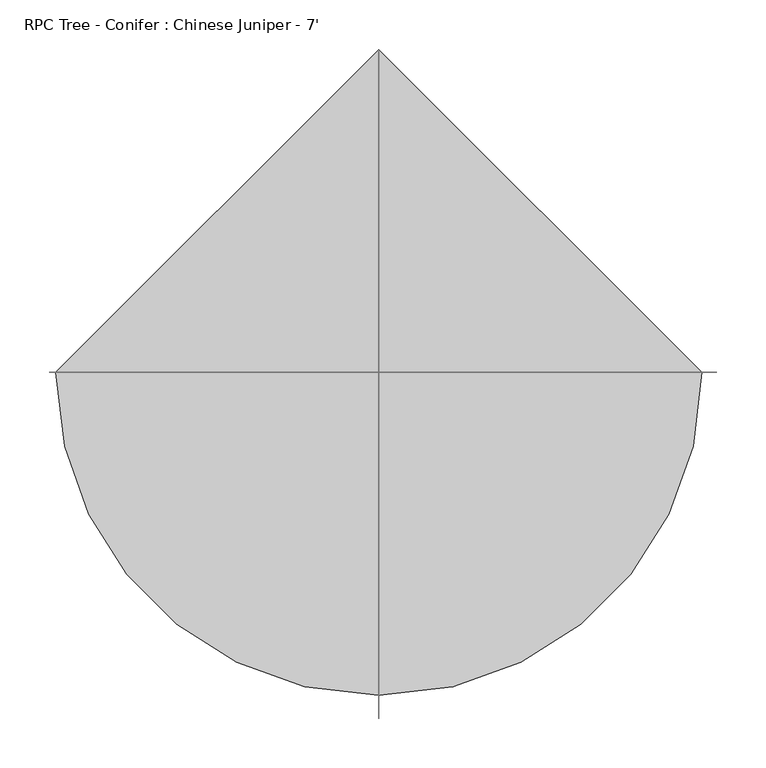
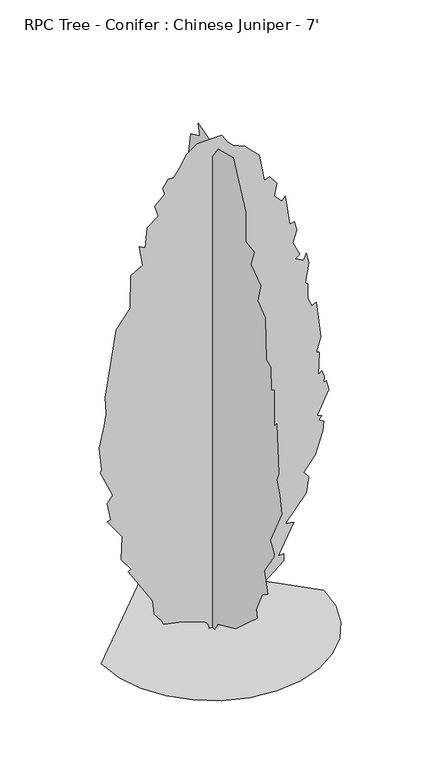
"""IFC4 building model written with IfcOpenShell, lengths in millimetres: geographic element geometry, RPC Tree - Conifer : Chinese Juniper - 7'."""

from ifc_helpers import new_model, si_unit, origin, place, context, project, spatial, triangles, source, transform, mapped, element, save


def rpc_tree_conifer_chinese_juniper_7_7598bbdc(model_context):
    return source(origin(), model_context, "Body", "Tessellation", [
        triangles([(-10.3135556, 5e-07, 9e-07), (-12.8060293, -2e-07, 12.8140684), (-19.5312093, -4e-07, 21.7081794), (-88.2070433, 1.1e-06, 46.9827109), (-143.9981418, 2.8e-06, 58.8213279), (-149.3455807, 2.2e-06, 72.1897524), (-170.8912042, 1.5e-06, 99.7706089), (-176.0828022, -7e-07, 141.7057854), (-184.1045146, -1.3e-06, 157.7479294), (-248.2723821, -4.6e-06, 259.3475236), (-239.9701817, -5.3e-06, 264.3368267), (-268.362017, -6.4e-06, 304.1387577), (-265.4845582, -1.07e-05, 374.7346484), (-309.7677564, -1.24e-05, 435.812788), (-299.0725335, -1.31e-05, 438.4852266), (-309.3523021, -1.58e-05, 492.5148502), (-293.7240046, -1.78e-05, 513.3483533), (-331.1564581, -2.11e-05, 596.2342461), (-325.8097278, -2.16e-05, 601.5809764), (-333.8307135, -2.56e-05, 673.7698477), (-319.3200076, -2.99e-05, 736.7529219), (-312.4402313, -3.24e-05, 772.6976755), (-315.1144867, -3.53e-05, 823.4978451), (-283.0305802, -4.87e-05, 1024.024268), (-242.9256517, -5.36e-05, 1077.4986929), (-240.7575791, -5.96e-05, 1177.3046648), (-205.4931982, -6.24e-05, 1197.8151861), (-216.1884393, -6.56e-05, 1259.3087437), (-197.9348478, -6.58e-05, 1248.8367085), (-192.1255003, -6.97e-05, 1310.1089859), (-160.0402858, -7.25e-05, 1334.1719067), (-170.7351817, -7.41e-05, 1368.9301048), (-141.3244133, -7.7e-05, 1395.667281), (-146.6718613, -7.79e-05, 1414.3835804), (-130.6297082, -8e-05, 1438.4465012), (-114.5875642, -8.07e-05, 1438.4465012), (-96.1815747, -8.29e-05, 1462.3443157), (-77.7287857, -8.58e-05, 1497.0336227), (-44.6214088, -8.86e-05, 1519.4527485), (26.5664902, -9.18e-05, 1520.5723022), (43.1603652, -9.1e-05, 1494.5933647), (59.2025137, -9.07e-05, 1478.551466), (94.8687642, -9.14e-05, 1463.445702), (136.7395278, -9.06e-05, 1419.7303471), (152.7816628, -8.64e-05, 1336.846162), (168.8238158, -8.74e-05, 1342.1929287), (188.3895002, -8.66e-05, 1314.20205), (182.191877, -8.41e-05, 1278.0250431), (203.5823773, -8.36e-05, 1253.9621223), (214.2758017, -8.47e-05, 1264.6573997), (227.6453163, -7.99e-05, 1173.7504486), (241.0130141, -8.06e-05, 1176.424704), (248.2828829, -7.94e-05, 1149.9378759), (236.3339574, -7.67e-05, 1113.592202), (257.0549855, -7.5e-05, 1069.4776709), (243.0450304, -7.39e-05, 1061.0775295), (267.7502266, -7.42e-05, 1048.0871887), (275.7712123, -7.56e-05, 1066.8034155), (283.792198, -7.41e-05, 1034.7194727), (273.0987737, -7.01e-05, 975.8983538), (280.8185786, -7.01e-05, 969.5464886), (279.746333, -6.74e-05, 926.116), (291.8131837, -6.63e-05, 898.3609354), (305.1827165, -6.72e-05, 903.7077021), (318.5503962, -6.11e-05, 791.4139023), (305.1827165, -5.8e-05, 748.6347548), (313.5084801, -5.81e-05, 745.8062937), (310.5294468, -5.39e-05, 676.4441031), (321.2246879, -5.48e-05, 684.4650524), (329.2456736, -5.41e-05, 665.7488256), (326.5713819, -5.28e-05, 647.0344156), (334.5923676, -5.33e-05, 649.7068542), (342.6133533, -5.19e-05, 620.2971668), (307.8551551, -4.63e-05, 550.7808068), (321.2246879, -4.65e-05, 545.4340765), (313.2037022, -4.56e-05, 534.7388354), (326.5713819, -4.57e-05, 526.7178497), (323.7592352, -4.38e-05, 497.9014764), (302.5084248, -3.89e-05, 430.4642409), (267.7502266, -3.48e-05, 387.6850571), (283.792198, -3.44e-05, 368.9688303), (275.0237288, -3.12e-05, 322.2617249), (214.2758017, -2.4e-05, 245.9798258), (238.3405755, -2.49e-05, 243.3055704), (192.8871181, -1.77e-05, 155.0742009), (208.9290895, -1.84e-05, 155.0742009), (208.9290895, -1.71e-05, 133.684618), (91.2864429, -6.2e-06, 37.4317359), (91.2864429, -7e-06, 50.8001605), (11.0759977, -5e-07, 0.0), (0.1966718, 9.8494079, 9.29e-05), (0.1966729, 24.6293697, 10.2116678), (0.1966747, 55.3021477, 21.3897713), (0.1966762, 127.4919001, 48.1266227), (0.1966794, 164.923636, 82.8846392), (0.1966788, 148.881492, 85.5583586), (0.1966849, 206.1035171, 168.0404152), (0.1966859, 188.9874833, 208.5473722), (0.1966882, 237.1133793, 278.0637686), (0.1966893, 231.7666672, 310.147675), (0.1966927, 266.5230486, 352.9268589), (0.1966955, 278.2089087, 404.0935395), (0.1966947, 271.8715775, 457.2014534), (0.1966993, 314.6507795, 521.369339), (0.1967023, 317.3232182, 585.539005), (0.1967039, 301.8799747, 638.0518244), (0.1967057, 325.3442039, 721.897506), (0.1967061, 303.9555203, 751.3071934), (0.1967086, 277.2183078, 836.8655611), (0.1967091, 295.9345346, 895.68668), (0.1967119, 274.5440343, 981.2450478), (0.196713, 247.8086386, 1032.0452173), (0.1967142, 234.439124, 1138.9940672), (0.1967132, 218.3971526, 1130.9731178), (0.1967174, 218.3971526, 1227.2249462), (0.1967163, 186.3132279, 1235.2458229), (0.1967152, 169.3394457, 1292.3597786), (0.1967168, 159.5761971, 1339.5204174), (0.1967168, 127.4919001, 1371.6043602), (0.1967204, 111.449747, 1467.8579327), (0.1967164, 65.9968483, 1489.2467434), (0.1967182, 72.8998653, 1523.6638287), (0.1967145, 8.1062543, 1503.0081127), (0.1967152, 4.5019648, 1457.1628006), (0.1967129, -27.5823121, 1502.6161308), (0.1967105, -105.1193285, 1524.0049416), (0.1967048, -169.2880862, 1392.9930256), (0.1967008, -169.2880862, 1302.0879639), (0.1966987, -211.5754214, 1294.5605164), (0.1966973, -193.3508616, 1245.9411003), (0.1966964, -244.8876323, 1210.7601809), (0.1966946, -230.7833333, 1155.0360386), (0.1966917, -268.2139701, 1125.6245344), (0.1966887, -273.562499, 997.2870192), (0.1966873, -295.3920532, 987.9742882), (0.1966841, -297.6254561, 917.0771622), (0.1966839, -313.6674093, 927.7706228), (0.1966819, -313.6674093, 815.4768957), (0.1966791, -327.0351254, 831.5188671), (0.196675, -337.7303664, 681.7926138), (0.1966744, -326.120719, 656.3254183), (0.1966719, -343.0789135, 617.6229115), (0.1966721, -351.0998629, 564.1485229), (0.1966695, -294.9511826, 449.1804677), (0.1966673, -313.6674093, 417.0965612), (0.1966698, -312.0853475, 405.769927), (0.1966688, -262.8672579, 334.2124489), (0.1966653, -281.5834847, 272.7170382), (0.1966657, -252.1719987, 254.0008115), (0.1966671, -222.7623476, 189.8329441), (0.1966658, -228.1090598, 165.7690968), (0.196666, -174.6353615, 117.6426557), (0.1966663, -118.4877531, 66.8424907), (0.1966685, -24.9082271, 24.0633114), (0.1966709, -11.5401454, 9.16e-05), (-327.063394, 0.0, 0.0001066), (-318.4110515, -74.9863023, 0.0001017), (-293.7711855, -143.8493682, 9.65e-05), (-255.1158779, -204.615799, 9.12e-05), (-204.4191359, -255.312541, 8.6e-05), (-143.652696, -293.9678487, 8.1e-05), (-74.7896301, -318.6077328, 7.66e-05), (0.1966858, -327.2600753, 7.28e-05), (75.1829745, -318.6077328, 7e-05), (144.0460404, -293.9678487, 6.85e-05), (204.8124621, -255.312541, 6.81e-05), (255.5092041, -204.615799, 6.89e-05), (294.1645118, -143.8491865, 7.08e-05), (318.8044141, -74.9863023, 7.39e-05), (327.4567566, 2.86e-05, 7.8e-05), (0.1966283, 327.2600753, 0.0001118)], [[57, 58, 59], [27, 28, 29], [87, 88, 89], [49, 50, 51], [13, 14, 15], [83, 84, 85], [74, 75, 76], [63, 64, 65], [68, 69, 70], [71, 72, 73], [9, 10, 11], [85, 86, 87], [85, 87, 89], [51, 52, 53], [54, 55, 56], [90, 1, 2], [66, 67, 68], [45, 46, 47], [17, 18, 19], [68, 70, 71], [45, 47, 48], [31, 32, 33], [76, 77, 78], [89, 90, 2], [89, 2, 3], [57, 59, 60], [51, 53, 54], [25, 26, 27], [39, 40, 41], [56, 57, 60], [71, 73, 74], [34, 35, 36], [33, 34, 36], [4, 5, 6], [60, 61, 62], [80, 81, 82], [38, 39, 41], [37, 38, 41], [37, 41, 42], [29, 30, 31], [15, 16, 17], [36, 37, 42], [33, 36, 42], [31, 33, 42], [31, 42, 43], [31, 43, 44], [31, 44, 45], [29, 31, 45], [29, 45, 48], [27, 29, 48], [25, 27, 48], [25, 48, 49], [25, 49, 51], [25, 51, 54], [25, 54, 56], [25, 56, 60], [25, 60, 62], [24, 25, 62], [23, 24, 62], [22, 23, 62], [22, 62, 63], [22, 63, 65], [22, 65, 66], [22, 66, 68], [21, 22, 68], [20, 21, 68], [19, 20, 68], [17, 19, 68], [17, 68, 71], [17, 71, 74], [15, 17, 74], [13, 15, 74], [13, 74, 76], [13, 76, 78], [13, 78, 79], [13, 79, 80], [12, 13, 80], [11, 12, 80], [9, 11, 80], [9, 80, 82], [9, 82, 83], [9, 83, 85], [9, 85, 89], [9, 89, 3], [9, 3, 4], [8, 9, 4], [8, 4, 6], [7, 8, 6], [138, 139, 140], [94, 95, 96], [136, 137, 138], [121, 122, 123], [112, 113, 114], [128, 129, 130], [121, 123, 124], [125, 126, 127], [124, 125, 127], [114, 115, 116], [147, 148, 149], [130, 131, 132], [124, 127, 128], [134, 135, 136], [154, 155, 91], [154, 91, 92], [150, 151, 152], [96, 97, 98], [119, 120, 121], [119, 121, 124], [119, 124, 128], [118, 119, 128], [117, 118, 128], [116, 117, 128], [116, 128, 130], [114, 116, 130], [114, 130, 132], [112, 114, 132], [112, 132, 133], [112, 133, 134], [112, 134, 136], [111, 112, 136], [110, 111, 136], [109, 110, 136], [109, 136, 138], [109, 138, 140], [109, 140, 141], [108, 109, 141], [107, 108, 141], [106, 107, 141], [105, 106, 141], [104, 105, 141], [103, 104, 141], [103, 141, 142], [103, 142, 143], [103, 143, 144], [102, 103, 144], [101, 102, 144], [100, 101, 144], [100, 144, 145], [100, 145, 146], [100, 146, 147], [100, 147, 149], [100, 149, 150], [100, 150, 152], [100, 152, 153], [100, 153, 154], [99, 100, 154], [98, 99, 154], [96, 98, 154], [96, 154, 92], [96, 92, 93], [96, 93, 94], [170, 171, 156], [169, 170, 156], [169, 156, 157], [168, 169, 157], [168, 157, 158], [168, 158, 159], [167, 168, 159], [166, 167, 159], [166, 159, 160], [166, 160, 161], [166, 161, 162], [166, 162, 163], [166, 163, 164], [166, 164, 165]], closed=False),
    ])


if __name__ == "__main__":
    model = new_model("IFC4")
    model_context = context("Model", 3, world=origin())
    ifc_project = project(units=[si_unit("LENGTHUNIT", "METRE", prefix="MILLI")], contexts=[model_context])
    site = spatial("IfcSite", under=ifc_project)
    building = spatial("IfcBuilding", under=site)
    placement = place(None, origin())
    rpc_tree_conifer_chinese_juniper_7_shape = rpc_tree_conifer_chinese_juniper_7_7598bbdc(model_context)
    element("IfcGeographicElement", 1, ObjectType="RPC Tree - Conifer : Chinese Juniper - 7'", at=placement, inside=building, context=model_context, shape_type="MappedRepresentation", body=[
        mapped(rpc_tree_conifer_chinese_juniper_7_shape, transform((0.0, 0.0, 0.0), x_axis=(1.0, 0.0, 0.0), y_axis=(0.0, 1.0, 0.0), z_axis=(0.0, 0.0, 1.0))),
    ])
    save(model, "model.ifc")

# Revit data of these elements
# Type "RPC Tree - Conifer : Chinese Juniper - 7'"
#   built-in parameter 1005198 = "{2, 15},{39, RPC-16-FUM3-UUQ0-UBF0-N000-ST1L-LVER-AU},{1, 0},{1, 0},{2, 13},{1, 8},{5, Color},{1, 0},{1, 0},{3, 0.8},{3, 0.8},{3, 0.8},{1, 8},{7, BBoxMin},{1, 0},{1, 0},{1, 0},{1, 0},{1, 0},{1, 8},{7, BBoxMax},{1, 0},{1, 0},{1, 0},{1, 0},{1, 0},{2, 11},{9, RPCTypeId},{1, 0},{1, 0},{39, RPC-16-FUM3-UUQ0-UBF0-N000-ST1L-LVER-AU},{1, 6},{14, RPCPlantHeight},{1, 0},{1, 0},{1, 7},{2, 11},{7, keyword},{1, 0},{1, 0},{34, :RPCs:Trees [General]:Geometry:RPC},{2, 11},{8, category},{1, 0},{1, 0},{15, Trees [General]},{2, 11},{12, LocalizedUID},{1, 0},{1, 0},{15, Chinese Juniper},{2, 14},{6, Height},{1, 0},{1, 0},{1, 7},{1, 2},{16, Cast Reflections},{1, 0},{1, 0},{1, 0},{1, 2},{12, Cast Shadows},{1, 0},{1, 0},{1, 1},{1, 2},{9, Lock View},{1, 0},{1, 0},{1, 0},{1, 4},{5, ViewC},{1, 0},{1, 0},{1, 0},{21, assetlibrary_base.fbx},{1, 5},"
#   built-in parameter 1005195 = "RPC-16-FUM3-UUQ0-UBF0-N000-ST1L-LVER-AU"
#   Type Comments = "Chinese Juniper"
#   Assembly Code = "G2050500"
#   Height = 5' - 0"
#   Description = (empty or 0)
#   Default Elevation = 0
